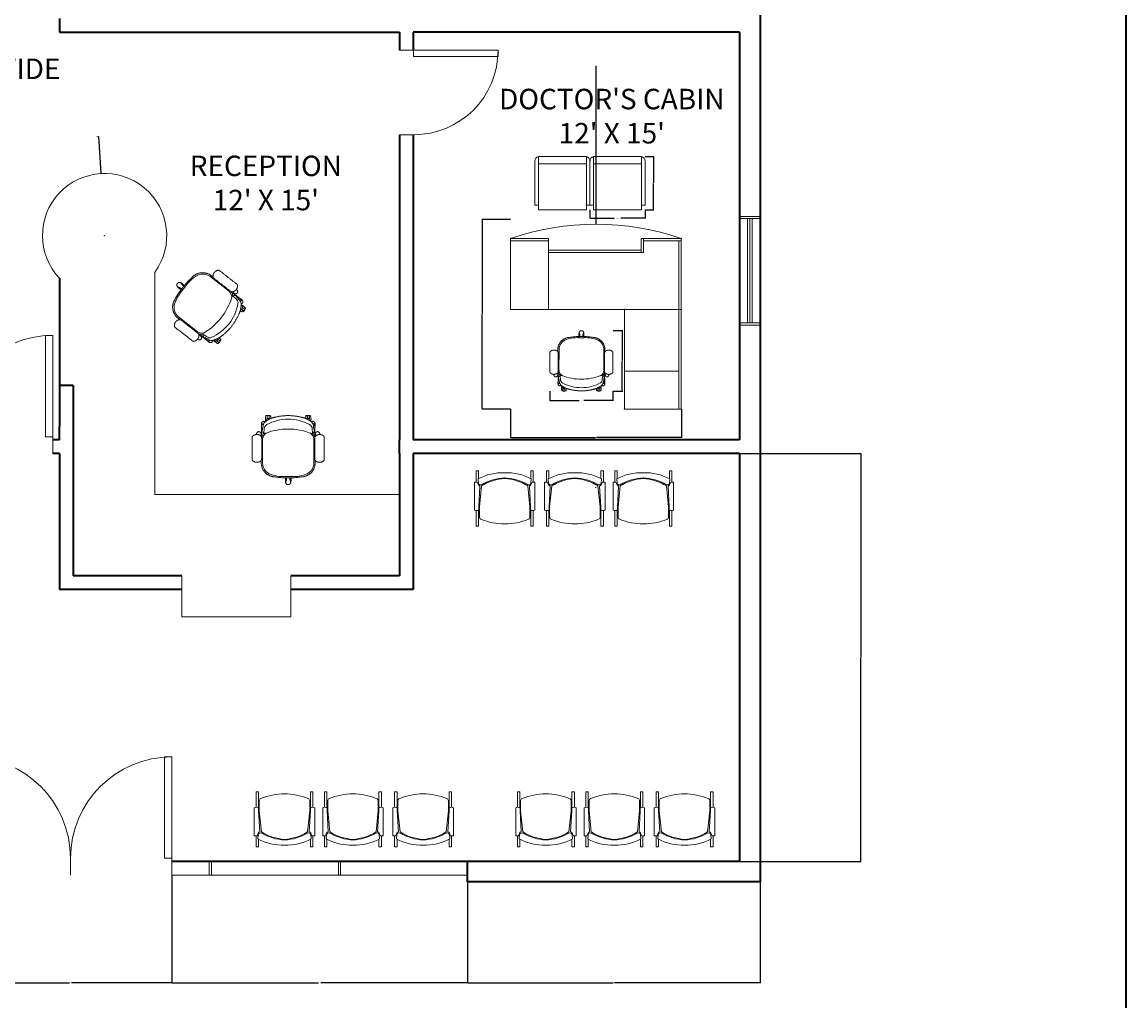
# Model space of a CAD drawing. Units: inches. Extents: x 7245 to 8143, y 15548 to 17244.
# Tile 3 of 5: x 7657 to 8143, y 15902 to 16334. Entities that reach past the tile are written whole.
import ezdxf

# ---------------------------------------------------------------- set-up
doc = ezdxf.new("R2010")
doc.units = ezdxf.units.IN
for name, color, linetype, lineweight in [('A-ANNO-DIMS', 2, 'Continuous', 18), ('A-ANNO-TTLB', 7, 'Continuous', 35), ('A-AREA-IDEN', 7, 'Continuous', 18), ('A-DOOR', 3, 'Continuous', 18), ('A-FLOR-CASE', 9, 'Continuous', 20), ('A-FURN', 8, 'Continuous', 18), ('A-GLAZ', 4, 'Continuous', 18), ('A-WALL', 7, 'Continuous', 35)]:
    doc.layers.add(name, color=color, linetype=linetype, lineweight=lineweight)
doc.styles.get("Standard").update_dxf_attribs({"font": 'arial.ttf'})
doc.dimstyles.get("Standard").update_dxf_attribs({"dimtxt": 0.18, "dimasz": 0.18, "dimexe": 0.18, "dimexo": 0.0625, "dimgap": 0.09, "dimtad": 0, "dimtih": 1, "dimtoh": 1, "dimdec": 4, "dimzin": 0, "dimdsep": 46, "dimtxsty": 'Standard', "dimcen": 0.09, "dimadec": 0, "dimazin": 0, "dimtfac": 1, "dimtdec": 4, "dimtofl": 0, "dimtmove": 0, "dimatfit": 3, "dimfxl": 1, "dimtolj": 1, "dimtzin": 0, "dimarcsym": 0})

# ---------------------------------------------------------------- blocks, each defined once
blk = doc.blocks.new('*U2')
for p, q in [((-600, 0), (-600, 100)), ((0, 0), (0, 100))]:
    blk.add_line(p, q)
blk.add_lwpolyline([(0, 0), (0, -600), (-43.75, -600), (-43.75, 0)], close=True)
blk.add_arc((0, 0), 600, 180, 270)
blk = doc.blocks.new('fdss')
at = {"color": 0}
for p, q in [((426, 240), (196, 239)), ((470, 236), (480, 226)), ((480, 225), (479, 223)), ((482, 204), (480, 210)), ((484, 228), (520, 224)), ((617, 196), (646, 196)), ((618, 179), (646, 179)), ((647, 195), (647, 179)), ((482, -204), (480, -210)), ((617, -196), (646, -196)), ((618, -179), (646, -179)), ((647, -195), (647, -179)), ((426, -240), (196, -239)), ((470, -236), (480, -226)), ((480, -225), (479, -223)), ((484, -228), (520, -224))]:
    blk.add_line(p, q, dxfattribs=at)
for points in [[(505, 245), (520, 247), (546, 249), (551, 249)], [(566, 236), (554, 235), (512, 240)], [(33, 21), (34, 20), (36, 19), (37, 18), (37, 18), (39, 18)], [(39, 18), (41, 17), (43, 17), (46, 16), (47, 16), (50, 16), (53, 16), (55, 16), (57, 16), (60, 16), (63, 16)], [(75, -28), (75, 0), (75, 28)], [(33, -21), (34, -20), (36, -19), (37, -18), (37, -18), (39, -18)], [(39, -18), (41, -17), (43, -17), (46, -16), (47, -16), (50, -16), (53, -16), (55, -16), (57, -16), (60, -16), (63, -16)], [(505, -245), (520, -247), (546, -249), (551, -249)], [(566, -236), (554, -235), (512, -240)]]:
    blk.add_lwpolyline(points, dxfattribs=at)
at = {"color": 0, "extrusion": (0, 0, -1)}
for centre, major_axis, start_param, end_param in [((201, 128), (-79, 79), 5.969012, 7.027382), ((424, 173), (47, 47), -0.751727, 0.301996), ((424, 175), (54.1, 54.1), -0.544214, -0.156468), ((514, 220), (24.9, 24.9), 3.662908, 4.015109), ((484, 224), (3.3, 3.3), 4.243712, 5.205719), ((484, 229), (-1.47, 1.47), 3.927418, 5.578652), ((500, 224), (-12.9, 12.9), 5.819354, 6.506047), ((509, 207), (26.9, 26.9), -1.329065, -0.883773), ((521, 177), (-33.1, 33.1), 0.763307, 1.830683), ((550, 228), (14.8, 14.8), -0.735707, 0.161366), ((545, 180), (-39.3, 39.3), 0.935679, 1.762262), ((566, 238), (1.31, 1.31), 0.929037, 2.293349), ((563, 238), (-2.9, 2.9), 1.793197, 2.458506), ((597, 186), (15.6, 15.6), -0.947253, 1.474381), ((445, 42), (-262, 262), 5.459154, 5.874691), ((-41, 3), (553, 91), -0.204201, 0.167634), ((193, 0), (-296, 296), 1.856147, 2.355859), ((621, 198), (-1.12, 1.12), 2.396655, 3.926991), ((621, 177), (-1.12, 1.12), 0.785398, 2.315734), ((646, 195), (0.539, 0.539), -0.785398, 0.785398), ((646, 179), (-0.539, 0.539), 2.356195, 3.926991)]:
    blk.add_ellipse(centre, major_axis=major_axis, ratio=1, start_param=start_param, end_param=end_param, dxfattribs=at)
at = {"color": 0}
for centre, major_axis, start_param, end_param in [((445, -42), (262, 262), 2.317561, 2.733098), ((-41, -3), (-553, 91), 2.937392, 3.309227), ((193, 0), (296, 296), 4.99774, 5.497452), ((201, -128), (79, 79), 2.82742, 3.885789), ((424, -173), (-47, 47), 2.389866, 3.443588), ((521, -177), (33.1, 33.1), 3.9049, 4.972275), ((597, -186), (15.6, 15.6), 3.765136, 6.18677), ((621, -177), (1.12, 1.12), 3.926991, 5.457327), ((621, -198), (1.12, 1.12), 5.538248, 7.068583), ((646, -179), (0.539, 0.539), 5.497787, 7.068583), ((646, -195), (-0.539, 0.539), 2.356195, 3.926991), ((424, -175), (-54.1, 54.1), 2.597378, 2.985125), ((514, -220), (-24.9, 24.9), 0.521315, 0.873517), ((484, -224), (-3.3, 3.3), 1.102119, 2.064126), ((484, -229), (1.47, 1.47), 0.785825, 2.437059), ((500, -224), (12.9, 12.9), 2.677762, 3.364454), ((509, -207), (-26.9, 26.9), 1.812527, 2.25782), ((550, -228), (-14.8, 14.8), 2.405886, 3.302959), ((545, -180), (39.3, 39.3), 4.077272, 4.903855), ((566, -238), (-1.31, 1.31), 4.07063, 5.434941), ((563, -238), (2.9, 2.9), 4.93479, 5.600098)]:
    blk.add_ellipse(centre, major_axis=major_axis, ratio=1, start_param=start_param, end_param=end_param, dxfattribs=at)
for points, weights, knots in [([(436, 337), (338, 337), (240, 337), (234, 338), (228, 335), (217, 328), (212, 315), (204, 293), (212, 271), (217, 258), (228, 251), (234, 248), (240, 248)], [1, 1, 1, 0.962754439438, 1, 0.939418827348, 1, 0.934055427035, 1, 0.939418827348, 1, 0.962754439438, 1], [0, 0, 0, 1, 1, 1.54757, 1.54757, 2.247301, 2.247301, 2.977684, 2.977684, 3.677415, 3.677415, 4.224984, 4.224984, 4.224984]), ([(436, 337), (443, 338), (449, 335), (460, 328), (464, 315), (473, 293), (464, 271), (460, 258), (449, 251), (443, 248), (436, 248), (338, 248), (240, 248)], [1, 0.96275443944, 1, 0.939418827348, 1, 0.934055427035, 1, 0.939418827348, 1, 0.96275443944, 1, 1, 1], [0, 0, 0, 0.54757, 0.54757, 1.247301, 1.247301, 1.977684, 1.977684, 2.677415, 2.677415, 3.224984, 3.224984, 4.224984, 4.224984, 4.224984]), ([(227, 252), (219, 252), (211, 252), (156, 255), (115, 218), (74, 180), (72, 125), (63, 75), (63, 25), (63, 13), (62, 0), (63, -13), (63, -25), (63, -75), (72, -125), (74, -180), (115, -218), (156, -255), (211, -252), (219, -252), (227, -252)], [1, 1, 1, 0.920970329426, 1, 0.920970329426, 1, 0.996764637726, 1, 1, 1, 1, 1, 0.996764637726, 1, 0.920970329426, 1, 0.920970329426, 1, 1, 1], [0, 0, 0, 1, 1, 1.800466, 1.800466, 2.600931, 2.600931, 2.761856, 2.761856, 3.761856, 3.761856, 4.761856, 4.761856, 4.922781, 4.922781, 5.723247, 5.723247, 6.523712, 6.523712, 7.523712, 7.523712, 7.523712]), ([(447, 248), (506, 249), (566, 251), (577, 251), (585, 244), (591, 239), (592, 232), (592, 228), (590, 225), (589, 221), (585, 219)], [1, 1, 1, 0.935512434708, 1, 0.918468104225, 1, 0.965843473499, 1, 0.972653000165, 1], [0, 0, 0, 1, 1, 1.722179, 1.722179, 2.535393, 2.535393, 3.059628, 3.059628, 3.528435, 3.528435, 3.528435]), ([(468, 296), (480, 296), (489, 288), (493, 285), (494, 280), (496, 274), (494, 268), (488, 255), (474, 254), (463, 254), (452, 253)], [1, 0.943338632687, 1, 0.968267368414, 1, 0.9394851057, 1, 0.864198855487, 1, 1, 1], [0, 0, 0, 0.676489, 0.676489, 1.181677, 1.181677, 1.881021, 1.881021, 2.935502, 2.935502, 3.935502, 3.935502, 3.935502]), ([(591, 211), (619, 173), (629, 128), (645, 65), (645, 0), (645, -65), (629, -128), (619, -173), (591, -211)], [1, 0.979760898136, 1, 0.992391068779, 1, 0.992391068779, 1, 0.979760898136, 1], [0, 0, 0, 0.403066, 0.403066, 0.649944, 0.649944, 0.896822, 0.896822, 1.299888, 1.299888, 1.299888]), ([(592, 211), (618, 216), (643, 209), (646, 209), (646, 206), (646, 203), (646, 199), (646, 198), (644, 198), (630, 198), (616, 198)], [1, 0.974666881773, 1, 0.783317345499, 1, 1, 1, 0.707106807826, 1, 1, 1], [0, 0, 0, 0.451139, 0.451139, 1.792762, 1.792762, 2.792762, 2.792762, 4.363559, 4.363559, 5.363559, 5.363559, 5.363559]), ([(618, 177), (631, 177), (644, 177), (645, 177), (645, 176), (646, 176), (646, 175), (646, 172), (646, 168), (646, 166), (643, 165), (631, 161), (619, 161)], [1, 1, 1, 0.923879528314, 1, 0.923879528314, 1, 1, 1, 0.783317456604, 1, 0.992237440768, 1], [0, 0, 0, 1, 1, 1.785398, 1.785398, 2.570796, 2.570796, 3.570796, 3.570796, 4.912419, 4.912419, 5.161781, 5.161781, 5.161781]), ([(33, -20), (22, -27), (10, -20), (-1, -13), (0, 0), (-1, 13), (10, 20), (22, 27), (33, 20)], [1, 0.85579821339, 1, 0.85579821339, 1, 0.855798213391, 1, 0.855798213391, 1], [0, 0, 0, 1.087409, 1.087409, 2.174818, 2.174818, 3.262227, 3.262227, 4.349636, 4.349636, 4.349636]), ([(12, 21), (13, 23), (15, 23), (39, 29), (63, 25)], [1, 0.873023611703, 1, 0.980536821249, 1], [0, 0, 0, 1.018856, 1.018856, 1.414094, 1.414094, 1.414094]), ([(12, -21), (13, -23), (15, -23), (39, -29), (63, -25)], [1, 0.873023611717, 1, 0.980536821249, 1], [0, 0, 0, 1.018856, 1.018856, 1.414094, 1.414094, 1.414094]), ([(592, -211), (618, -216), (643, -209), (646, -209), (646, -206), (646, -203), (646, -199), (646, -198), (644, -198), (630, -198), (616, -198)], [1, 0.974666881774, 1, 0.7833173455, 1, 1, 1, 0.707106807832, 1, 1, 1], [0, 0, 0, 0.451139, 0.451139, 1.792762, 1.792762, 2.792762, 2.792762, 4.363559, 4.363559, 5.363559, 5.363559, 5.363559]), ([(618, -177), (631, -177), (644, -177), (645, -177), (645, -176), (646, -176), (646, -175), (646, -172), (646, -168), (646, -166), (643, -165), (631, -161), (619, -161)], [1, 1, 1, 0.923879528318, 1, 0.923879528318, 1, 1, 1, 0.783317456602, 1, 0.992237440768, 1], [0, 0, 0, 1, 1, 1.785398, 1.785398, 2.570796, 2.570796, 3.570796, 3.570796, 4.912419, 4.912419, 5.161781, 5.161781, 5.161781]), ([(464, -271), (460, -258), (449, -251), (443, -248), (436, -248), (338, -248), (240, -248), (234, -248), (228, -251), (217, -258), (212, -271), (204, -293), (212, -315), (217, -328), (228, -335), (234, -338), (240, -337), (338, -337), (436, -337)], [1, 0.939418827349, 1, 0.96275443944, 1, 1, 1, 0.962754439438, 1, 0.939418827349, 1, 0.934055427035, 1, 0.939418827348, 1, 0.962754439438, 1, 1, 1], [0, 0, 0, 0.699731, 0.699731, 1.247301, 1.247301, 2.247301, 2.247301, 2.794871, 2.794871, 3.494602, 3.494602, 4.224984, 4.224984, 4.924715, 4.924715, 5.472285, 5.472285, 6.472285, 6.472285, 6.472285]), ([(464, -271), (473, -293), (464, -315), (460, -328), (449, -335), (443, -338), (436, -337)], [1, 0.934055427035, 1, 0.939418827348, 1, 0.96275443944, 1], [0, 0, 0, 0.730383, 0.730383, 1.430114, 1.430114, 1.977684, 1.977684, 1.977684]), ([(447, -248), (506, -249), (566, -251), (577, -251), (585, -244), (591, -239), (592, -232), (592, -228), (590, -225), (589, -221), (585, -219)], [1, 1, 1, 0.935512434708, 1, 0.918468104224, 1, 0.965843473499, 1, 0.972653000166, 1], [0, 0, 0, 1, 1, 1.722179, 1.722179, 2.535393, 2.535393, 3.059628, 3.059628, 3.528435, 3.528435, 3.528435]), ([(468, -296), (480, -296), (489, -288), (493, -285), (494, -280), (496, -274), (494, -268), (488, -255), (474, -254), (463, -254), (452, -253)], [1, 0.943338632687, 1, 0.968267368413, 1, 0.9394851057, 1, 0.864198855486, 1, 1, 1], [0, 0, 0, 0.676489, 0.676489, 1.181677, 1.181677, 1.881021, 1.881021, 2.935502, 2.935502, 3.935502, 3.935502, 3.935502])]:
    blk.add_rational_spline(points, weights, degree=2, knots=knots, dxfattribs=at)
blk = doc.blocks.new('*U5')
for p, q in [((-600, 0), (-600, -100)), ((0, 0), (0, -100))]:
    blk.add_line(p, q)
blk.add_lwpolyline([(0, 0), (0, 600), (-43.75, 600), (-43.75, 0)], close=True)
blk.add_arc((0, 0), 600, 90, 180)
blk = doc.blocks.new('chair033')
at = {"color": 0, "lineweight": -2}
for points in [[(-230, -108.2), (-230, 16.8), (-210, 16.8), (-210, -113.2)], [(230, -108.2), (230, 16.8), (210, 16.8), (210, -113.2)], [(-230, -338.2), (-230, -428.2), (-210, -428.2), (-210, -365.9)], [(230, -338.2), (230, -428.2), (210, -428.2), (210, -365.9)]]:
    blk.add_lwpolyline(points, dxfattribs=at)
for points in [[(1.1, -366.9, -0.129806), (-186.5, -306.8), (-203.9, -137.4), (-203.9, -55.9, -0.30894), (-191.2, -37.2, -0.09648), (0, 0, -0.09648)], [(-1.1, -366.9, 0.129806), (186.5, -306.8), (203.9, -137.4), (203.9, -55.9, 0.30894), (191.2, -37.2, 0.09648), (0, 0, 0.09648)], [(1.1, -371.9, -0.119401), (-186.5, -316.8, 0.398658), (-212.2, -326.8), (-215, -363.2, 0.13244), (0, -413.2)], [(-1.1, -371.9, 0.119401), (186.5, -316.8, -0.398658), (212.2, -326.8), (215, -363.2, -0.13244), (0, -413.2)]]:
    blk.add_lwpolyline(points, format="xyb", dxfattribs=at)
for points in [[(-243.9, -337.4), (-243.9, -157.4), (-243.9, -112.4, -0.285714), (-208.9, -112.4), (-208.9, -137.4), (-199.3, -306, 0.220172), (-212.2, -316.8), (-221.9, -337.4)], [(243.9, -337.4), (243.9, -157.4), (243.9, -112.4, 0.285714), (208.9, -112.4), (208.9, -137.4), (199.3, -306, -0.220172), (212.2, -316.8), (221.9, -337.4)]]:
    blk.add_lwpolyline(points, format="xyb", close=True, dxfattribs=at)
blk = doc.blocks.new('dfgdddd')
at = {"color": 0, "ltscale": 10}
for p, q in [((-295, 522), (-295, 51)), ((-257, 0), (-257, 571)), ((-257, 571), (257, 571)), ((257, 494), (-257, 494)), ((257, 571), (257, 0)), ((295, 522), (295, 51)), ((-295, 51), (-257, 51)), ((257, 0), (-257, 0)), ((295, 51), (257, 51))]:
    blk.add_line(p, q, dxfattribs=at)
for centre, start, end in [((-244, 522), 104.4775, 180), ((244, 522), 0, 75.5225)]:
    blk.add_arc(centre, 50.8, start, end, dxfattribs=at)
blk = doc.blocks.new('table directors')
at = {"color": 0}
for p, q in [((151.60625, 914.4), (913.60625, 914.4)), ((151.60625, 482.6), (151.60625, 914.4)), ((177.00625, 914.4), (177.00625, 508)), ((177.00625, 889), (913.60625, 889)), ((913.60625, 914.4), (913.60625, -914.4)), ((1980.40625, 914.4), (913.60625, 914.4)), ((913.60625, 914.4), (913.60625, 304.8)), ((1980.40625, 889), (913.60625, 889)), ((1574.00625, 304.8), (1574.00625, 889)), ((1980.40625, 304.8), (1980.40625, 914.4)), ((151.60625, 508), (304.00625, 508)), ((151.60625, 482.6), (304.00625, 482.6)), ((278.60625, -508), (278.60625, 482.6)), ((304.00625, 508), (304.00625, -508)), ((913.60625, 304.8), (1980.40625, 304.8)), ((1980.40625, 304.8), (1574.00625, 304.8)), ((913.60625, -508), (151.60625, -508)), ((151.60625, -914.4), (151.60625, -508)), ((177.00625, -508), (177.00625, -914.4)), ((913.60625, -914.4), (913.60625, -508)), ((913.60625, -914.4), (151.60625, -914.4)), ((329.40625, -914.4), (913.60625, -914.4))]:
    blk.add_line(p, q, dxfattribs=at)
blk.add_arc((2819.4, 0), 2819.4, 161.075358315, 198.924646694, dxfattribs=at)
for p in [(151.60625, 912.8125), (913.60625, 914.4), (913.60625, 914.4), (1980.40625, 914.4), (913.60625, 304.8), (1980.40625, 304.8), (151.60625, -914.4), (913.60625, -914.4)]:
    blk.add_point(p, dxfattribs=at)
at = {"color": 0, "text_generation_flag": 4, "flags": 1}
for tag in ['CAPGC', 'CAPDH', 'CAPQT', 'CAPMC', 'CAPMG', 'CAPPN']:
    blk.add_attdef(tag, (913.60625, 914.4), '', height=0.0254, rotation=270, dxfattribs=at)
at = {"color": 0, "flags": 1}
for tag in ['CAPMG', 'CAPMC', 'CAPDH', 'CAPQT', 'CAPGC', 'CAPPN']:
    blk.add_attdef(tag, (151.60625, -914.4), '', height=0.0254, rotation=90, dxfattribs=at)
blk = doc.blocks.new('*D28')
at = {"layer": 'A-ANNO-DIMS', "color": 0, "lineweight": -2, "transparency": 16777216}
for p, q in [((7889.41, 16170.73), (7889.41, 16166.45)), ((7917.19, 16170.73), (7917.19, 16166.45)), ((7889.59, 16166.63), (7902.28, 16166.63)), ((7917.01, 16166.63), (7904.31, 16166.63))]:
    blk.add_line(p, q, dxfattribs=at)
at = {"layer": 'A-ANNO-DIMS', "color": 0, "transparency": 16777216}
for points in [[(7889.59, 16166.66), (7889.59, 16166.6), (7889.41, 16166.63)], [(7917.01, 16166.66), (7917.01, 16166.6), (7917.19, 16166.63)]]:
    blk.add_solid(points, dxfattribs=at)
at = {"layer": 'Defpoints', "color": 0, "transparency": 16777216}
for p in [(7889.41, 16170.8), (7917.19, 16170.8), (7889.41, 16166.63)]:
    blk.add_point(p, dxfattribs=at)
at = {"layer": 'A-ANNO-DIMS', "color": 0, "transparency": 16777216, "insert": (7903.3, 16166.63), "char_height": 0.18, "attachment_point": 5}
blk.add_mtext('\\A1;DESK CHAIR 28', dxfattribs=at)
blk = doc.blocks.new('*D29')
at = {"layer": 'A-ANNO-DIMS', "color": 0, "lineweight": -2, "transparency": 16777216}
for p, q in [((7917.25, 16197.43), (7921.53, 16197.43)), ((7921.35, 16197.25), (7921.35, 16184.29)), ((7921.35, 16170.98), (7921.35, 16183.93)), ((7917.25, 16170.8), (7921.53, 16170.8))]:
    blk.add_line(p, q, dxfattribs=at)
at = {"layer": 'A-ANNO-DIMS', "color": 0, "transparency": 16777216}
for points in [[(7921.32, 16197.25), (7921.38, 16197.25), (7921.35, 16197.43)], [(7921.32, 16170.98), (7921.38, 16170.98), (7921.35, 16170.8)]]:
    blk.add_solid(points, dxfattribs=at)
at = {"layer": 'Defpoints', "color": 0, "transparency": 16777216}
for p in [(7917.19, 16197.43), (7917.19, 16170.8), (7921.35, 16170.8)]:
    blk.add_point(p, dxfattribs=at)
at = {"layer": 'A-ANNO-DIMS', "color": 0, "transparency": 16777216, "insert": (7921.35, 16184.11), "char_height": 0.18, "attachment_point": 5}
blk.add_mtext('\\A1;27', dxfattribs=at)
blk = doc.blocks.new('*D34')
at = {"layer": 'A-ANNO-DIMS', "color": 0, "lineweight": -2, "transparency": 16777216}
for p, q in [((7907.07, 16250.71), (7907.07, 16246.94)), ((7931.39, 16250.71), (7931.39, 16246.94)), ((7907.25, 16247.12), (7917.81, 16247.12)), ((7931.21, 16247.12), (7920.65, 16247.12))]:
    blk.add_line(p, q, dxfattribs=at)
at = {"layer": 'A-ANNO-DIMS', "color": 0, "transparency": 16777216}
for points in [[(7907.25, 16247.15), (7907.25, 16247.09), (7907.07, 16247.12)], [(7931.21, 16247.15), (7931.21, 16247.09), (7931.39, 16247.12)]]:
    blk.add_solid(points, dxfattribs=at)
at = {"layer": 'Defpoints', "color": 0, "transparency": 16777216}
for p in [(7907.07, 16250.77), (7931.39, 16250.77), (7931.39, 16247.12)]:
    blk.add_point(p, dxfattribs=at)
at = {"layer": 'A-ANNO-DIMS', "color": 0, "transparency": 16777216, "insert": (7919.23, 16247.12), "char_height": 0.18, "attachment_point": 5}
blk.add_mtext('\\A1;GUEST CHAIR 24 TYP.', dxfattribs=at)
blk = doc.blocks.new('*D35')
at = {"layer": 'A-ANNO-DIMS', "color": 0, "lineweight": -2, "transparency": 16777216}
for p, q in [((7931.45, 16274.3), (7935.22, 16274.3)), ((7935.04, 16274.12), (7935.04, 16262.72)), ((7935.04, 16250.95), (7935.04, 16262.36)), ((7931.45, 16250.77), (7935.22, 16250.77))]:
    blk.add_line(p, q, dxfattribs=at)
at = {"layer": 'A-ANNO-DIMS', "color": 0, "transparency": 16777216}
for points in [[(7935.01, 16274.12), (7935.07, 16274.12), (7935.04, 16274.3)], [(7935.01, 16250.95), (7935.07, 16250.95), (7935.04, 16250.77)]]:
    blk.add_solid(points, dxfattribs=at)
at = {"layer": 'Defpoints', "color": 0, "transparency": 16777216}
for p in [(7931.39, 16274.3), (7935.04, 16274.3), (7931.39, 16250.77)]:
    blk.add_point(p, dxfattribs=at)
at = {"layer": 'A-ANNO-DIMS', "color": 0, "transparency": 16777216, "insert": (7935.04, 16262.54), "char_height": 0.18, "attachment_point": 5}
blk.add_mtext('\\A1;24 TYP.', dxfattribs=at)
blk = doc.blocks.new('*D40')
at = {"layer": 'A-ANNO-DIMS', "color": 0, "lineweight": -2, "transparency": 16777216}
for p, q in [((7872.01, 16246.49), (7859.35, 16246.49)), ((7859.53, 16246.31), (7859.53, 16204.85)), ((7859.53, 16163.03), (7859.53, 16204.49)), ((7872.01, 16162.85), (7859.35, 16162.85))]:
    blk.add_line(p, q, dxfattribs=at)
at = {"layer": 'A-ANNO-DIMS', "color": 0, "transparency": 16777216}
for points in [[(7859.5, 16246.31), (7859.56, 16246.31), (7859.53, 16246.49)], [(7859.5, 16163.03), (7859.56, 16163.03), (7859.53, 16162.85)]]:
    blk.add_solid(points, dxfattribs=at)
at = {"layer": 'Defpoints', "color": 0, "transparency": 16777216}
for p in [(7872.07, 16246.49), (7859.53, 16162.85), (7872.07, 16162.85)]:
    blk.add_point(p, dxfattribs=at)
at = {"layer": 'A-ANNO-DIMS', "color": 0, "transparency": 16777216, "insert": (7859.53, 16204.67), "char_height": 0.18, "attachment_point": 5}
blk.add_mtext('\\A1;OFFICE DESK 84', dxfattribs=at)
blk = doc.blocks.new('*D41')
at = {"layer": 'A-ANNO-DIMS', "color": 0, "lineweight": -2, "transparency": 16777216}
for p, q in [((7872.07, 16162.79), (7872.07, 16150.13)), ((7947.38, 16162.79), (7947.38, 16150.13)), ((7872.25, 16150.31), (7909.5, 16150.31)), ((7947.2, 16150.31), (7909.94, 16150.31))]:
    blk.add_line(p, q, dxfattribs=at)
at = {"layer": 'A-ANNO-DIMS', "color": 0, "transparency": 16777216}
for points in [[(7872.25, 16150.34), (7872.25, 16150.28), (7872.07, 16150.31)], [(7947.2, 16150.34), (7947.2, 16150.28), (7947.38, 16150.31)]]:
    blk.add_solid(points, dxfattribs=at)
at = {"layer": 'Defpoints', "color": 0, "transparency": 16777216}
for p in [(7872.07, 16162.85), (7947.38, 16162.85), (7947.38, 16150.31)]:
    blk.add_point(p, dxfattribs=at)
at = {"layer": 'A-ANNO-DIMS', "color": 0, "transparency": 16777216, "insert": (7909.72, 16150.31), "char_height": 0.18, "attachment_point": 5}
blk.add_mtext('\\A1;75', dxfattribs=at)
blk = doc.blocks.new('*D46')
at = {"layer": 'A-ANNO-DIMS', "color": 0, "lineweight": -2, "transparency": 16777216}
for p, q in [((7633.26, 15957.13), (7633.26, 15909.51)), ((7722.64, 15957.13), (7722.64, 15909.51)), ((7633.44, 15909.69), (7677.55, 15909.69)), ((7722.46, 15909.69), (7678.34, 15909.69))]:
    blk.add_line(p, q, dxfattribs=at)
at = {"layer": 'A-ANNO-DIMS', "color": 0, "transparency": 16777216}
for points in [[(7633.44, 15909.72), (7633.44, 15909.66), (7633.26, 15909.69)], [(7722.46, 15909.72), (7722.46, 15909.66), (7722.64, 15909.69)]]:
    blk.add_solid(points, dxfattribs=at)
at = {"layer": 'Defpoints', "color": 0, "transparency": 16777216}
for p in [(7633.26, 15957.19), (7722.64, 15957.19), (7722.64, 15909.69)]:
    blk.add_point(p, dxfattribs=at)
at = {"layer": 'A-ANNO-DIMS', "color": 0, "transparency": 16777216, "insert": (7677.95, 15909.69), "char_height": 0.18, "attachment_point": 5}
blk.add_mtext('\\A1;89.37', dxfattribs=at)
blk = doc.blocks.new('*D47')
at = {"layer": 'A-ANNO-DIMS', "color": 0, "lineweight": -2, "transparency": 16777216}
for p, q in [((7722.64, 15957.13), (7722.64, 15909.51)), ((7853.08, 15957.13), (7853.08, 15909.51)), ((7722.82, 15909.69), (7787.4, 15909.69)), ((7852.9, 15909.69), (7788.32, 15909.69))]:
    blk.add_line(p, q, dxfattribs=at)
at = {"layer": 'A-ANNO-DIMS', "color": 0, "transparency": 16777216}
for points in [[(7722.82, 15909.72), (7722.82, 15909.66), (7722.64, 15909.69)], [(7852.9, 15909.72), (7852.9, 15909.66), (7853.08, 15909.69)]]:
    blk.add_solid(points, dxfattribs=at)
at = {"layer": 'Defpoints', "color": 0, "transparency": 16777216}
for p in [(7722.64, 15957.19), (7853.08, 15957.19), (7853.08, 15909.69)]:
    blk.add_point(p, dxfattribs=at)
at = {"layer": 'A-ANNO-DIMS', "color": 0, "transparency": 16777216, "insert": (7787.86, 15909.69), "char_height": 0.18, "attachment_point": 5}
blk.add_mtext('\\A1;130.45', dxfattribs=at)
blk = doc.blocks.new('*D48')
at = {"layer": 'A-ANNO-DIMS', "color": 0, "lineweight": -2, "transparency": 16777216}
for p, q in [((7853.08, 15954.13), (7853.08, 15909.51)), ((7982.08, 15954.13), (7982.08, 15909.51)), ((7853.26, 15909.69), (7917.3, 15909.69)), ((7981.9, 15909.69), (7917.86, 15909.69))]:
    blk.add_line(p, q, dxfattribs=at)
at = {"layer": 'A-ANNO-DIMS', "color": 0, "transparency": 16777216}
for points in [[(7853.26, 15909.72), (7853.26, 15909.66), (7853.08, 15909.69)], [(7981.9, 15909.72), (7981.9, 15909.66), (7982.08, 15909.69)]]:
    blk.add_solid(points, dxfattribs=at)
at = {"layer": 'Defpoints', "color": 0, "transparency": 16777216}
for p in [(7853.08, 15954.19), (7982.08, 15954.19), (7982.08, 15909.69)]:
    blk.add_point(p, dxfattribs=at)
at = {"layer": 'A-ANNO-DIMS', "color": 0, "transparency": 16777216, "insert": (7917.58, 15909.69), "char_height": 0.18, "attachment_point": 5}
blk.add_mtext('\\A1;129', dxfattribs=at)
blk = doc.blocks.new('*D49')
at = {"layer": 'A-ANNO-DIMS', "color": 0, "lineweight": -2, "transparency": 16777216}
for p, q in [((7973.15, 16143.19), (8026.76, 16143.19)), ((8026.58, 16143.01), (8026.58, 16053.37)), ((8026.58, 15963.37), (8026.58, 16053.01)), ((7973.15, 15963.19), (8026.76, 15963.19))]:
    blk.add_line(p, q, dxfattribs=at)
at = {"layer": 'A-ANNO-DIMS', "color": 0, "transparency": 16777216}
for points in [[(8026.55, 16143.01), (8026.61, 16143.01), (8026.58, 16143.19)], [(8026.55, 15963.37), (8026.61, 15963.37), (8026.58, 15963.19)]]:
    blk.add_solid(points, dxfattribs=at)
at = {"layer": 'Defpoints', "color": 0, "transparency": 16777216}
for p in [(7973.08, 16143.19), (8026.58, 16143.19), (7973.08, 15963.19)]:
    blk.add_point(p, dxfattribs=at)
at = {"layer": 'A-ANNO-DIMS', "color": 0, "transparency": 16777216, "insert": (8026.58, 16053.19), "char_height": 0.18, "attachment_point": 5}
blk.add_mtext('\\A1;180', dxfattribs=at)
blk = doc.blocks.new('*D79')
at = {"layer": 'A-ANNO-DIMS', "color": 0, "lineweight": -2, "transparency": 16777216}
for p, q in [((7690.05, 16283.17), (7690.23, 16283.17)), ((7690.23, 16283.17), (7691.25, 16266.93)), ((7692.89, 16239.38), (7693.07, 16239.38)), ((7692.98, 16239.29), (7692.98, 16239.47))]:
    blk.add_line(p, q, dxfattribs=at)
at = {"layer": 'A-ANNO-DIMS', "color": 0, "transparency": 16777216}
blk.add_solid([(7691.28, 16266.93), (7691.22, 16266.92), (7691.26, 16266.75)], dxfattribs=at)
at = {"layer": 'Defpoints', "color": 0, "transparency": 16777216}
for p in [(7691.26, 16266.75), (7692.98, 16239.38)]:
    blk.add_point(p, dxfattribs=at)
at = {"layer": 'A-ANNO-DIMS', "color": 0, "transparency": 16777216, "insert": (7689.57, 16283.17), "char_height": 0.18, "attachment_point": 5}
blk.add_mtext('\\A1;R27.42', dxfattribs=at)
blk = doc.blocks.new('*D80')
at = {"layer": 'A-ANNO-DIMS', "color": 0, "lineweight": -2, "transparency": 16777216}
for p, q in [((7909.9, 16314.05), (7909.72, 16314.05)), ((7909.72, 16314.05), (7909.72, 16244.58)), ((7909.63, 16128.31), (7909.81, 16128.31)), ((7909.72, 16128.22), (7909.72, 16128.4))]:
    blk.add_line(p, q, dxfattribs=at)
at = {"layer": 'A-ANNO-DIMS', "color": 0, "transparency": 16777216}
blk.add_solid([(7909.69, 16244.58), (7909.75, 16244.58), (7909.72, 16244.4)], dxfattribs=at)
at = {"layer": 'Defpoints', "color": 0, "transparency": 16777216}
for p in [(7909.72, 16244.4), (7909.72, 16128.31)]:
    blk.add_point(p, dxfattribs=at)
at = {"layer": 'A-ANNO-DIMS', "color": 0, "transparency": 16777216, "insert": (7910.37, 16314.05), "char_height": 0.18, "attachment_point": 5}
blk.add_mtext('\\A1;R116.1', dxfattribs=at)

msp = doc.modelspace()

# ---------------------------------------------------------------- linework, layer by layer
at = {"layer": 'A-ANNO-TTLB'}
msp.add_lwpolyline([(7245.2864, 17243.9412), (8143.486, 17243.9412), (8143.486, 15548.1459), (7245.2864, 15548.1459)], close=True, dxfattribs=at)
at = {"layer": 'A-FLOR-CASE'}
for p, q in [((7715.0838, 16125.1899), (7715.0838, 16223.1591)), ((7823.0838, 16125.1899), (7715.0838, 16125.1899)), ((7727.0838, 16071.1899), (7727.0838, 16089.1899)), ((7775.0838, 16089.1899), (7775.0838, 16071.1899)), ((7775.0838, 16071.1899), (7727.0838, 16071.1899))]:
    msp.add_line(p, q, dxfattribs=at)
msp.add_arc((7692.9819, 16239.3835), 27.4176, 323.71862, 223.46918, dxfattribs=at)
at = {"layer": 'A-GLAZ'}
for p, q in [((7982.0838, 16247.8711), (7973.0838, 16247.8711)), ((7973.0838, 16247.8711), (7973.0838, 16199.8711)), ((7982.0838, 16246.8711), (7973.0838, 16246.8711)), ((7976.5838, 16200.8711), (7976.5838, 16246.8711)), ((7977.5838, 16200.8711), (7977.5838, 16246.8711)), ((7978.5838, 16200.8711), (7978.5838, 16246.8711)), ((7982.0838, 16199.8711), (7982.0838, 16247.8711)), ((7973.0838, 16200.8711), (7982.0838, 16200.8711)), ((7973.0838, 16199.8711), (7982.0838, 16199.8711)), ((7739.0838, 15957.1899), (7739.0838, 15963.1899)), ((7740.0838, 15957.1899), (7740.0838, 15963.1899)), ((7796.0838, 15957.1899), (7796.0838, 15963.1899)), ((7797.0838, 15957.1899), (7797.0838, 15963.1899)), ((7722.6356, 15957.1899), (7853.0838, 15957.1899))]:
    msp.add_line(p, q, dxfattribs=at)
at = {"layer": 'A-WALL'}
for p, q in [((7982.0838, 16842.1899), (7982.0838, 15954.1899)), ((7673.0838, 16335.1899), (7673.0838, 16329.1899)), ((7673.0838, 16329.1899), (7823.0838, 16329.1899)), ((7823.0838, 16329.1899), (7823.0838, 16321.144)), ((7973.0838, 16329.1899), (7829.0838, 16329.1899)), ((7829.0838, 16329.1899), (7829.0838, 16321.144)), ((7973.0838, 16329.1899), (7973.0838, 16149.1899)), ((7823.0838, 16283.884), (7823.0838, 16149.1899)), ((7823.0838, 16283.884), (7823.0838, 16149.1899)), ((7823.0838, 16283.884), (7823.0838, 16149.1899)), ((7829.0838, 16283.884), (7829.0838, 16149.1899)), ((7673.0838, 16220.5212), (7673.0838, 16155.1899)), ((7679.0838, 16173.2922), (7673.0838, 16173.2922)), ((7679.0838, 16173.2922), (7679.0838, 16089.1899)), ((7673.0838, 16149.1899), (7673.0838, 16155.1899)), ((7673.0838, 16149.1899), (7670.1656, 16149.1899)), ((7823.0838, 16143.1899), (7823.0838, 16149.1899)), ((7973.0838, 16149.1899), (7829.0838, 16149.1899)), ((7673.0838, 16143.1899), (7670.1656, 16143.1899)), ((7673.0838, 16143.1899), (7673.0838, 16083.1899)), ((7823.0838, 16143.1899), (7823.0838, 16089.1899)), ((7973.0838, 16143.1899), (7829.0838, 16143.1899)), ((7973.0838, 16143.1899), (7829.0838, 16143.1899)), ((7829.0838, 16143.1899), (7829.0838, 16083.1899)), ((7973.0838, 16143.1899), (7973.0838, 15963.1899)), ((7727.0838, 16089.1899), (7679.0838, 16089.1899)), ((7823.0838, 16089.1899), (7775.0838, 16089.1899)), ((7727.0838, 16083.1899), (7673.0838, 16083.1899)), ((7829.0838, 16083.1899), (7775.0838, 16083.1899)), ((7973.0838, 15963.1899), (7722.6356, 15963.1899)), ((7853.0838, 15954.1899), (7853.0838, 15963.1899)), ((7982.0838, 15954.1899), (7853.0838, 15954.1899))]:
    msp.add_line(p, q, dxfattribs=at)

# ---------------------------------------------------------------- block references
at = {"layer": 'A-DOOR'}
for name, p, xscale, yscale, zscale, rotation in [('*U5', (7829.2938, 16321.144), -0.0620999814668474, 0.0620999814668474, 0.0620999814668474, 270), ('*U2', (7670.1656, 16150.6378), -0.0744787106297815, 0.0744787106297815, 0.0744787106297815, 180), ('*U2', (7633.2612, 15964.6378), 0.0744787106297815, 0.0744787106297815, 0.0744787106297815, 180), ('*U2', (7722.6356, 15964.6378), -0.0744787106297815, 0.0744787106297815, 0.0744787106297815, 180)]:
    msp.add_blockref(name, p, dxfattribs=dict(at, xscale=xscale, yscale=yscale, zscale=zscale, rotation=rotation))
at = {"layer": 'A-FURN'}
for name, p, xscale, yscale, zscale in [('dfgdddd', (7894.9138, 16250.7725), -0.0411765943226869, 0.0411765943226869, 0.0411765943226869), ('dfgdddd', (7919.2307, 16250.7725), 0.0411765943226869, 0.0411765943226869, 0.0411765943226869), ('chair033', (7772.3347, 15993.0101), 0.0546397566719344, 0.0546397566719344, 0.0546397566719344), ('chair033', (7802.5249, 15993.0101), 0.0546397566719344, 0.0546397566719344, 0.0546397566719344), ('chair033', (7833.4892, 15993.0101), 0.0546397566719344, 0.0546397566719344, 0.0546397566719344), ('chair033', (7887.6357, 15993.0101), 0.0546397566719344, 0.0546397566719344, 0.0546397566719344), ('chair033', (7917.8259, 15993.0101), 0.0546397566719344, 0.0546397566719344, 0.0546397566719344), ('chair033', (7948.7902, 15993.0101), 0.0546397566719344, 0.0546397566719344, 0.0546397566719344)]:
    msp.add_blockref(name, p, dxfattribs=dict(at, xscale=xscale, yscale=yscale, zscale=zscale))
for name, p, xscale, yscale, zscale, rotation in [('table directors', (7909.7238, 16244.3983), 0.0411765943226869, 0.0411765943226869, 0.0411765943226869, 270), ('fdss', (7725.1228, 16218.2375), -0.0471859915129668, 0.0471859915129668, 0.0471859915129668, 141.9976487829288), ('fdss', (7903.297, 16197.4241), -0.0411765943226869, 0.0411765943226869, 0.0411765943226869, 90), ('fdss', (7773.9742, 16129.5085), -0.0471859915129668, 0.0471859915129668, 0.0471859915129668, 269.9947245832753), ('chair033', (7869.4571, 16112.1453), 0.0546397566719344, 0.0546397566719344, 0.0546397566719344, 180), ('chair033', (7900.4214, 16112.1453), 0.0546397566719344, 0.0546397566719344, 0.0546397566719344, 180), ('chair033', (7930.6116, 16112.1453), 0.0546397566719344, 0.0546397566719344, 0.0546397566719344, 180)]:
    msp.add_blockref(name, p, dxfattribs=dict(at, xscale=xscale, yscale=yscale, zscale=zscale, rotation=rotation))

# ---------------------------------------------------------------- texts
at = {"layer": 'A-AREA-IDEN', "char_height": 9.045999, "attachment_point": 1}
for s, insert in [("\\pxqc;{\\fArial|b1|i0|c0|p34;8' PASSAGE WIDE}", (7563.7227, 16317.5022)), ("\\pxqc;{\\fArial|b1|i0|c0|p34;DOCTOR'S CABIN^J12' X 15'}", (7856.587, 16304.1548)), ("\\pxqc;{\\fArial|b1|i0|c0|p34;RECEPTION ^J12' X 15'}", (7703.9987, 16274.6635))]:
    msp.add_mtext_dynamic_manual_height_columns(s, width=120.239684, gutter_width=18.8458, heights=[0], dxfattribs=dict(at, insert=insert))

# ---------------------------------------------------------------- dimensions: what is measured, and where the dimension line sits
at = {"layer": 'A-ANNO-DIMS'}
for center, mpoint, override, picture, middle in [((7909.7238, 16128.305), (7909.724, 16244.3983), {"dimdec": 1, "dimlfac": 1, "dimrnd": 0, "dimzin": 0, "dimdsep": 46, "dimlunit": 2}, '*D80', (7910.3666, 16314.0543)), ((7692.9819, 16239.3835), (7691.263, 16266.7471), {"dimdec": 2, "dimlfac": 1, "dimrnd": 0, "dimzin": 0, "dimdsep": 46, "dimlunit": 2}, '*D79', (7689.5727, 16283.1652))]:
    dim = msp.add_radius_dim(center=center, mpoint=mpoint, dimstyle='Standard', override=override, dxfattribs=at)
    dim.commit()
    dim.dimension.update_dxf_attribs({"geometry": picture, "text_midpoint": middle, "dimtype": 164})
for base, p1, p2, angle, text, picture, middle in [((7935.0366, 16274.3049), (7931.3891, 16250.7725), (7931.3891, 16274.3049), 90, '<> TYP.', '*D35', (7935.0366, 16262.5387)), ((7859.5261, 16162.8519), (7872.0719, 16246.4901), (7872.0719, 16162.8519), 270, 'OFFICE DESK <>', '*D40', (7859.5261, 16204.671)), ((7889.4061, 16166.6286), (7917.1869, 16170.7957), (7889.4061, 16170.7957), 180, 'DESK CHAIR <>', '*D28', (7903.2965, 16166.6286))]:
    dim = msp.add_linear_dim(base=base, p1=p1, p2=p2, angle=angle, text=text, dimstyle='Standard', override={"dimdec": 0, "dimlfac": 1, "dimrnd": 0, "dimzin": 0, "dimdsep": 46, "dimlunit": 2}, dxfattribs=at)
    dim.commit()
    dim.dimension.update_dxf_attribs({"geometry": picture, "text_midpoint": middle})
dim = msp.add_linear_dim(base=(7931.3891, 16247.1249), p1=(7907.0723, 16250.7725), p2=(7931.3891, 16250.7725), text='GUEST CHAIR <> TYP.', dimstyle='Standard', override={"dimdec": 0, "dimlfac": 1, "dimrnd": 0, "dimzin": 0, "dimdsep": 46, "dimlunit": 2}, dxfattribs=at)
dim.commit()
dim.dimension.update_dxf_attribs({"geometry": '*D34', "text_midpoint": (7919.2307, 16247.1249)})
for base, p1, p2, angle, picture, middle in [((7921.354, 16170.7957), (7917.1869, 16197.4266), (7917.1869, 16170.7957), 270, '*D29', (7921.354, 16184.1112)), ((8026.5838, 16143.1899), (7973.0838, 15963.1899), (7973.0838, 16143.1899), 90, '*D49', (8026.5838, 16053.1899))]:
    dim = msp.add_linear_dim(base=base, p1=p1, p2=p2, angle=angle, dimstyle='Standard', override={"dimdec": 0, "dimlfac": 1, "dimrnd": 0, "dimzin": 0, "dimdsep": 46, "dimlunit": 2}, dxfattribs=at)
    dim.commit()
    dim.dimension.update_dxf_attribs({"geometry": picture, "text_midpoint": middle})
for base, p1, p2, override, picture, middle in [((7947.3756, 16150.3062), (7872.0719, 16162.8519), (7947.3756, 16162.8519), {"dimdec": 0, "dimlfac": 1, "dimrnd": 0, "dimzin": 0, "dimdsep": 46, "dimlunit": 2}, '*D41', (7909.7237, 16150.3062)), ((7722.6356, 15909.6899), (7633.2612, 15957.1899), (7722.6356, 15957.1899), {"dimdec": 2, "dimlfac": 1, "dimrnd": 0, "dimzin": 0, "dimdsep": 46, "dimlunit": 2}, '*D46', (7677.9484, 15909.6899)), ((7853.0838, 15909.6899), (7722.6356, 15957.1899), (7853.0838, 15957.1899), {"dimdec": 2, "dimlfac": 1, "dimrnd": 0, "dimzin": 0, "dimdsep": 46, "dimlunit": 2}, '*D47', (7787.8597, 15909.6899)), ((7982.0838, 15909.6899), (7853.0838, 15954.1899), (7982.0838, 15954.1899), {"dimdec": 0, "dimlfac": 1, "dimrnd": 0, "dimzin": 0, "dimdsep": 46, "dimlunit": 2}, '*D48', (7917.5838, 15909.6899))]:
    dim = msp.add_linear_dim(base=base, p1=p1, p2=p2, dimstyle='Standard', override=override, dxfattribs=at)
    dim.commit()
    dim.dimension.update_dxf_attribs({"geometry": picture, "text_midpoint": middle})

doc.saveas('drawing.dxf')
